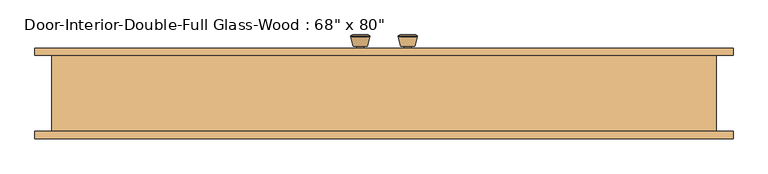
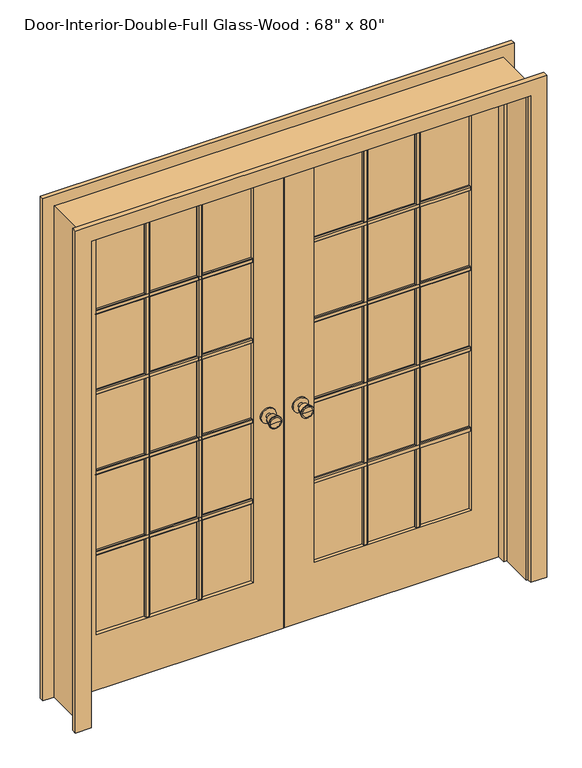
"""IFC4 building model written with IfcOpenShell, lengths in millimetres: door geometry."""

from ifc_helpers import new_model, si_unit, point, frame, frame_2d, origin, place, context, project, spatial, polyline, circle_curve, trimmed, segment, composite_curve, outline, extrude, faceted_brep, source, transform, mapped, element, save
from ifc_brep_helpers import plane_surface, cylinder_surface, revolved_surface, advanced_brep


def door_146fce4d(model_context):
    return source(origin(), model_context, "Body", "SolidModel", [
        advanced_brep(
        [(-63.5, 104.425, 914.4), (-73.5, 104.425, 914.4), (-53.5, 104.425, 914.4), (-83.9758676, 153.425, 914.4), (-63.5, 153.425, 914.4), (-43.0241324, 153.425, 914.4), (-88.5, 151.5971319, 914.4), (-38.5, 151.5971319, 914.4), (-88.5, 148.1334537, 914.4), (-38.5, 148.1334537, 914.4), (-82.136236, 123.425, 914.4), (-44.863764, 123.425, 914.4), (-73.5, 123.425, 914.4), (-53.5, 123.425, 914.4)],
        [
            (0, 1),
            (1, 2, circle_curve(frame((-63.5, 104.425, 914.4), z_axis=(0.0, -1.0, 0.0), x_axis=(1.0, 0.0, 0.0)), 10.0)),
            (2, 0),
            (2, 1, circle_curve(frame((-63.5, 104.425, 914.4), z_axis=(0.0, -1.0, 0.0), x_axis=(1.0, 0.0, 0.0)), 10.0)),
            (3, 4),
            (4, 5),
            (5, 3, circle_curve(frame((-63.5, 153.425, 914.4), z_axis=(0.0, 1.0, 0.0), x_axis=(1.0, 0.0, 0.0)), 20.4758676)),
            (3, 5, circle_curve(frame((-63.5, 153.425, 914.4), z_axis=(0.0, 1.0, 0.0), x_axis=(1.0, 0.0, 0.0)), 20.4758676)),
            (6, 3),
            (5, 7),
            (7, 6, circle_curve(frame((-63.5, 151.5971319, 914.4), z_axis=(0.0, 1.0, 0.0), x_axis=(1.0, 0.0, 0.0)), 25.0)),
            (6, 7, circle_curve(frame((-63.5, 151.5971319, 914.4), z_axis=(0.0, 1.0, 0.0), x_axis=(1.0, 0.0, 0.0)), 25.0)),
            (8, 6),
            (7, 9),
            (9, 8, circle_curve(frame((-63.5, 148.1334537, 914.4), z_axis=(0.0, 1.0, 0.0), x_axis=(1.0, 0.0, 0.0)), 25.0)),
            (8, 9, circle_curve(frame((-63.5, 148.1334537, 914.4), z_axis=(0.0, 1.0, 0.0), x_axis=(1.0, 0.0, 0.0)), 25.0)),
            (10, 8),
            (9, 11),
            (11, 10, circle_curve(frame((-63.5, 123.425, 914.4), z_axis=(0.0, 1.0, 0.0), x_axis=(1.0, 0.0, 0.0)), 18.636236)),
            (10, 11, circle_curve(frame((-63.5, 123.425, 914.4), z_axis=(0.0, 1.0, 0.0), x_axis=(1.0, 0.0, 0.0)), 18.636236)),
            (12, 10),
            (11, 13),
            (13, 12, circle_curve(frame((-63.5, 123.425, 914.4), z_axis=(0.0, 1.0, 0.0), x_axis=(1.0, 0.0, 0.0)), 10.0)),
            (12, 13, circle_curve(frame((-63.5, 123.425, 914.4), z_axis=(0.0, 1.0, 0.0), x_axis=(1.0, 0.0, 0.0)), 10.0)),
            (1, 12),
            (13, 2),
        ],
        [
            plane_surface(frame((-63.5, 104.425, 914.4), z_axis=(0.0, -1.0, 0.0), x_axis=(1.0, 0.0, 0.0))),
            plane_surface(frame((-63.5, 153.425, 914.4), z_axis=(0.0, 1.0, 0.0), x_axis=(1.0, 0.0, 0.0))),
            revolved_surface(polyline([(-43.0241324, 153.425, 914.4), (-38.5, 151.5971319, 914.4)]), (-63.5, 104.425, 914.4), (0.0, -1.0, 0.0)),
            cylinder_surface(frame((-63.5, 104.425, 914.4), z_axis=(0.0, -1.0, 0.0), x_axis=(1.0, 0.0, 0.0)), 25.0),
            revolved_surface(polyline([(-38.5, 148.1334537, 914.4), (-44.863764, 123.425, 914.4)]), (-63.5, 104.425, 914.4), (0.0, -1.0, 0.0)),
            plane_surface(frame((-63.5, 123.425, 914.4), z_axis=(0.0, -1.0, 0.0), x_axis=(1.0, 0.0, 0.0))),
            cylinder_surface(frame((-63.5, 104.425, 914.4), z_axis=(0.0, -1.0, 0.0), x_axis=(1.0, 0.0, 0.0)), 10.0),
        ],
        [
            (0, [[1, 2, 3]]),
            (0, [[-3, 4, -1]]),
            (1, [[5, 6, 7]]),
            (1, [[-6, -5, 8]]),
            (2, [[9, -7, 10, 11]]),
            (2, [[-10, -8, -9, 12]]),
            (3, [[13, -11, 14, 15]]),
            (3, [[-14, -12, -13, 16]]),
            (4, [[17, -15, 18, 19]]),
            (4, [[-18, -16, -17, 20]]),
            (5, [[21, -19, 22, 23]]),
            (5, [[-22, -20, -21, 24]]),
            (6, [[25, -23, 26, -2]]),
            (6, [[-26, -24, -25, -4]]),
        ],
    ),
        extrude(outline(composite_curve([segment(trimmed(circle_curve(frame_2d((914.4, -63.5)), 30.0), [point((914.4, -33.5))], [point((914.4, -93.5))], False, "CARTESIAN"), True, "CONTINUOUS"), segment(trimmed(circle_curve(frame_2d((914.4, -63.5)), 30.0), [point((914.4, -93.5))], [point((914.4, -33.5))], False, "CARTESIAN"), True, "CONTINUOUS")], self_intersect=False)), frame((0.0, 98.425, 0.0), z_axis=(0.0, 1.0, 0.0), x_axis=(0.0, 0.0, 1.0)), (0.0, 0.0, 1.0), 6.0),
        advanced_brep(
        [(-63.5, 57.5, 914.4), (-53.5, 57.5, 914.4), (-73.5, 57.5, 914.4), (-83.9758676, 8.5, 914.4), (-43.0241324, 8.5, 914.4), (-63.5, 8.5, 914.4), (-88.5, 10.3278681, 914.4), (-38.5, 10.3278681, 914.4), (-88.5, 13.7915463, 914.4), (-38.5, 13.7915463, 914.4), (-82.136236, 38.5, 914.4), (-44.863764, 38.5, 914.4), (-73.5, 38.5, 914.4), (-53.5, 38.5, 914.4)],
        [
            (0, 1),
            (1, 2, circle_curve(frame((-63.5, 57.5, 914.4), z_axis=(0.0, 1.0, 0.0), x_axis=(1.0, 0.0, 0.0)), 10.0)),
            (2, 0),
            (2, 1, circle_curve(frame((-63.5, 57.5, 914.4), z_axis=(0.0, 1.0, 0.0), x_axis=(1.0, 0.0, 0.0)), 10.0)),
            (3, 4, circle_curve(frame((-63.5, 8.5, 914.4), z_axis=(0.0, -1.0, 0.0), x_axis=(1.0, 0.0, 0.0)), 20.4758676)),
            (4, 5),
            (5, 3),
            (4, 3, circle_curve(frame((-63.5, 8.5, 914.4), z_axis=(0.0, -1.0, 0.0), x_axis=(1.0, 0.0, 0.0)), 20.4758676)),
            (6, 7, circle_curve(frame((-63.5, 10.3278681, 914.4), z_axis=(0.0, -1.0, 0.0), x_axis=(1.0, 0.0, 0.0)), 25.0)),
            (7, 4),
            (3, 6),
            (7, 6, circle_curve(frame((-63.5, 10.3278681, 914.4), z_axis=(0.0, -1.0, 0.0), x_axis=(1.0, 0.0, 0.0)), 25.0)),
            (8, 9, circle_curve(frame((-63.5, 13.7915463, 914.4), z_axis=(0.0, -1.0, 0.0), x_axis=(1.0, 0.0, 0.0)), 25.0)),
            (9, 7),
            (6, 8),
            (9, 8, circle_curve(frame((-63.5, 13.7915463, 914.4), z_axis=(0.0, -1.0, 0.0), x_axis=(1.0, 0.0, 0.0)), 25.0)),
            (10, 11, circle_curve(frame((-63.5, 38.5, 914.4), z_axis=(0.0, -1.0, 0.0), x_axis=(1.0, 0.0, 0.0)), 18.636236)),
            (11, 9),
            (8, 10),
            (11, 10, circle_curve(frame((-63.5, 38.5, 914.4), z_axis=(0.0, -1.0, 0.0), x_axis=(1.0, 0.0, 0.0)), 18.636236)),
            (12, 13, circle_curve(frame((-63.5, 38.5, 914.4), z_axis=(0.0, -1.0, 0.0), x_axis=(1.0, 0.0, 0.0)), 10.0)),
            (13, 11),
            (10, 12),
            (13, 12, circle_curve(frame((-63.5, 38.5, 914.4), z_axis=(0.0, -1.0, 0.0), x_axis=(1.0, 0.0, 0.0)), 10.0)),
            (1, 13),
            (12, 2),
        ],
        [
            plane_surface(frame((-63.5, 57.5, 914.4), z_axis=(0.0, 1.0, 0.0), x_axis=(1.0, 0.0, 0.0))),
            plane_surface(frame((-63.5, 8.5, 914.4), z_axis=(0.0, -1.0, 0.0), x_axis=(1.0, 0.0, 0.0))),
            revolved_surface(polyline([(-43.0241324, 8.5, 914.4), (-38.5, 10.3278681, 914.4)]), (-63.5, 57.5, 914.4), (0.0, 1.0, 0.0)),
            cylinder_surface(frame((-63.5, 57.5, 914.4), z_axis=(0.0, 1.0, 0.0), x_axis=(1.0, 0.0, 0.0)), 25.0),
            revolved_surface(polyline([(-38.5, 13.7915463, 914.4), (-44.863764, 38.5, 914.4)]), (-63.5, 57.5, 914.4), (0.0, 1.0, 0.0)),
            plane_surface(frame((-63.5, 38.5, 914.4), z_axis=(0.0, 1.0, 0.0), x_axis=(1.0, 0.0, 0.0))),
            cylinder_surface(frame((-63.5, 57.5, 914.4), z_axis=(0.0, 1.0, 0.0), x_axis=(1.0, 0.0, 0.0)), 10.0),
        ],
        [
            (0, [[1, 2, 3]]),
            (0, [[-3, 4, -1]]),
            (1, [[5, 6, 7]]),
            (1, [[8, -7, -6]]),
            (2, [[9, 10, -5, 11]]),
            (2, [[12, -11, -8, -10]]),
            (3, [[13, 14, -9, 15]]),
            (3, [[16, -15, -12, -14]]),
            (4, [[17, 18, -13, 19]]),
            (4, [[20, -19, -16, -18]]),
            (5, [[21, 22, -17, 23]]),
            (5, [[24, -23, -20, -22]]),
            (6, [[-2, 25, -21, 26]]),
            (6, [[-4, -26, -24, -25]]),
        ],
    ),
        extrude(outline(composite_curve([segment(trimmed(circle_curve(frame_2d((914.4, -63.5)), 30.0), [point((914.4, -33.5))], [point((914.4, -93.5))], False, "CARTESIAN"), True, "CONTINUOUS"), segment(trimmed(circle_curve(frame_2d((914.4, -63.5)), 30.0), [point((914.4, -93.5))], [point((914.4, -33.5))], False, "CARTESIAN"), True, "CONTINUOUS")], self_intersect=False)), frame((0.0, 57.5, 0.0), z_axis=(0.0, 1.0, 0.0), x_axis=(0.0, 0.0, 1.0)), (0.0, 0.0, 1.0), 6.0),
        extrude(outline(polyline([(77.47, 1586.23), (77.47, 1567.18), (71.12, 1567.18), (67.945, 1570.355), (67.945, 1583.055), (71.12, 1586.23), (77.47, 1586.23)])), frame((120.65, 0.0, 0.0), z_axis=(1.0, 0.0, 0.0), x_axis=(0.0, 1.0, 0.0)), (0.0, 0.0, 1.0), 622.3),
        extrude(outline(polyline([(77.47, 1249.9975), (77.47, 1230.9475), (71.12, 1230.9475), (67.945, 1234.1225), (67.945, 1246.8225), (71.12, 1249.9975), (77.47, 1249.9975)])), frame((120.65, 0.0, 0.0), z_axis=(1.0, 0.0, 0.0), x_axis=(0.0, 1.0, 0.0)), (0.0, 0.0, 1.0), 622.3),
        extrude(outline(polyline([(77.47, 913.765), (77.47, 894.715), (71.12, 894.715), (67.945, 897.89), (67.945, 910.59), (71.12, 913.765), (77.47, 913.765)])), frame((120.65, 0.0, 0.0), z_axis=(1.0, 0.0, 0.0), x_axis=(0.0, 1.0, 0.0)), (0.0, 0.0, 1.0), 622.3),
        extrude(outline(polyline([(77.47, 577.5325), (77.47, 558.4825), (71.12, 558.4825), (67.945, 561.6575), (67.945, 574.3575), (71.12, 577.5325), (77.47, 577.5325)])), frame((120.65, 0.0, 0.0), z_axis=(1.0, 0.0, 0.0), x_axis=(0.0, 1.0, 0.0)), (0.0, 0.0, 1.0), 622.3),
        extrude(outline(polyline([(525.9916667, 77.47), (545.0416667, 77.47), (545.0416667, 71.12), (541.8666667, 67.945), (529.1666667, 67.945), (525.9916667, 71.12), (525.9916667, 77.47)])), frame((0.0, 0.0, 231.775), z_axis=(0.0, 0.0, 1.0), x_axis=(1.0, 0.0, 0.0)), (0.0, 0.0, 1.0), 1681.1625),
        extrude(outline(polyline([(318.5583333, 77.47), (337.6083333, 77.47), (337.6083333, 71.12), (334.4333333, 67.945), (321.7333333, 67.945), (318.5583333, 71.12), (318.5583333, 77.47)])), frame((0.0, 0.0, 231.775), z_axis=(0.0, 0.0, 1.0), x_axis=(1.0, 0.0, 0.0)), (0.0, 0.0, 1.0), 1681.1625),
        extrude(outline(polyline([(84.455, 1586.23), (90.805, 1586.23), (93.98, 1583.055), (93.98, 1570.355), (90.805, 1567.18), (84.455, 1567.18), (84.455, 1586.23)])), frame((-742.95, 0.0, 0.0), z_axis=(1.0, 0.0, 0.0), x_axis=(0.0, 1.0, 0.0)), (0.0, 0.0, 1.0), 622.3),
        extrude(outline(polyline([(84.455, 1249.9975), (90.805, 1249.9975), (93.98, 1246.8225), (93.98, 1234.1225), (90.805, 1230.9475), (84.455, 1230.9475), (84.455, 1249.9975)])), frame((-742.95, 0.0, 0.0), z_axis=(1.0, 0.0, 0.0), x_axis=(0.0, 1.0, 0.0)), (0.0, 0.0, 1.0), 622.3),
        extrude(outline(polyline([(84.455, 913.765), (90.805, 913.765), (93.98, 910.59), (93.98, 897.89), (90.805, 894.715), (84.455, 894.715), (84.455, 913.765)])), frame((-742.95, 0.0, 0.0), z_axis=(1.0, 0.0, 0.0), x_axis=(0.0, 1.0, 0.0)), (0.0, 0.0, 1.0), 622.3),
        extrude(outline(polyline([(84.455, 577.5325), (90.805, 577.5325), (93.98, 574.3575), (93.98, 561.6575), (90.805, 558.4825), (84.455, 558.4825), (84.455, 577.5325)])), frame((-742.95, 0.0, 0.0), z_axis=(1.0, 0.0, 0.0), x_axis=(0.0, 1.0, 0.0)), (0.0, 0.0, 1.0), 622.3),
        extrude(outline(polyline([(-337.6083333, 84.455), (-337.6083333, 90.805), (-334.4333333, 93.98), (-321.7333333, 93.98), (-318.5583333, 90.805), (-318.5583333, 84.455), (-337.6083333, 84.455)])), frame((0.0, 0.0, 231.775), z_axis=(0.0, 0.0, 1.0), x_axis=(1.0, 0.0, 0.0)), (0.0, 0.0, 1.0), 1681.1625),
        extrude(outline(polyline([(-545.0416667, 84.455), (-545.0416667, 90.805), (-541.8666667, 93.98), (-529.1666667, 93.98), (-525.9916667, 90.805), (-525.9916667, 84.455), (-545.0416667, 84.455)])), frame((0.0, 0.0, 231.775), z_axis=(0.0, 0.0, 1.0), x_axis=(1.0, 0.0, 0.0)), (0.0, 0.0, 1.0), 1681.1625),
        extrude(outline(polyline([(84.455, 1586.23), (90.805, 1586.23), (93.98, 1583.055), (93.98, 1570.355), (90.805, 1567.18), (84.455, 1567.18), (84.455, 1586.23)])), frame((120.65, 0.0, 0.0), z_axis=(1.0, 0.0, 0.0), x_axis=(0.0, 1.0, 0.0)), (0.0, 0.0, 1.0), 622.3),
        extrude(outline(polyline([(84.455, 1249.9975), (90.805, 1249.9975), (93.98, 1246.8225), (93.98, 1234.1225), (90.805, 1230.9475), (84.455, 1230.9475), (84.455, 1249.9975)])), frame((120.65, 0.0, 0.0), z_axis=(1.0, 0.0, 0.0), x_axis=(0.0, 1.0, 0.0)), (0.0, 0.0, 1.0), 622.3),
        extrude(outline(polyline([(84.455, 913.765), (90.805, 913.765), (93.98, 910.59), (93.98, 897.89), (90.805, 894.715), (84.455, 894.715), (84.455, 913.765)])), frame((120.65, 0.0, 0.0), z_axis=(1.0, 0.0, 0.0), x_axis=(0.0, 1.0, 0.0)), (0.0, 0.0, 1.0), 622.3),
        extrude(outline(polyline([(84.455, 577.5325), (90.805, 577.5325), (93.98, 574.3575), (93.98, 561.6575), (90.805, 558.4825), (84.455, 558.4825), (84.455, 577.5325)])), frame((120.65, 0.0, 0.0), z_axis=(1.0, 0.0, 0.0), x_axis=(0.0, 1.0, 0.0)), (0.0, 0.0, 1.0), 622.3),
        extrude(outline(polyline([(525.9916667, 84.455), (525.9916667, 90.805), (529.1666667, 93.98), (541.8666667, 93.98), (545.0416667, 90.805), (545.0416667, 84.455), (525.9916667, 84.455)])), frame((0.0, 0.0, 231.775), z_axis=(0.0, 0.0, 1.0), x_axis=(1.0, 0.0, 0.0)), (0.0, 0.0, 1.0), 1681.1625),
        extrude(outline(polyline([(318.5583333, 84.455), (318.5583333, 90.805), (321.7333333, 93.98), (334.4333333, 93.98), (337.6083333, 90.805), (337.6083333, 84.455), (318.5583333, 84.455)])), frame((0.0, 0.0, 231.775), z_axis=(0.0, 0.0, 1.0), x_axis=(1.0, 0.0, 0.0)), (0.0, 0.0, 1.0), 1681.1625),
        extrude(outline(polyline([(77.47, 1586.23), (77.47, 1567.18), (71.12, 1567.18), (67.945, 1570.355), (67.945, 1583.055), (71.12, 1586.23), (77.47, 1586.23)])), frame((-742.95, 0.0, 0.0), z_axis=(1.0, 0.0, 0.0), x_axis=(0.0, 1.0, 0.0)), (0.0, 0.0, 1.0), 622.3),
        extrude(outline(polyline([(77.47, 1249.9975), (77.47, 1230.9475), (71.12, 1230.9475), (67.945, 1234.1225), (67.945, 1246.8225), (71.12, 1249.9975), (77.47, 1249.9975)])), frame((-742.95, 0.0, 0.0), z_axis=(1.0, 0.0, 0.0), x_axis=(0.0, 1.0, 0.0)), (0.0, 0.0, 1.0), 622.3),
        extrude(outline(polyline([(77.47, 913.765), (77.47, 894.715), (71.12, 894.715), (67.945, 897.89), (67.945, 910.59), (71.12, 913.765), (77.47, 913.765)])), frame((-742.95, 0.0, 0.0), z_axis=(1.0, 0.0, 0.0), x_axis=(0.0, 1.0, 0.0)), (0.0, 0.0, 1.0), 622.3),
        extrude(outline(polyline([(77.47, 577.5325), (77.47, 558.4825), (71.12, 558.4825), (67.945, 561.6575), (67.945, 574.3575), (71.12, 577.5325), (77.47, 577.5325)])), frame((-742.95, 0.0, 0.0), z_axis=(1.0, 0.0, 0.0), x_axis=(0.0, 1.0, 0.0)), (0.0, 0.0, 1.0), 622.3),
        extrude(outline(polyline([(-337.6083333, 77.47), (-318.5583333, 77.47), (-318.5583333, 71.12), (-321.7333333, 67.945), (-334.4333333, 67.945), (-337.6083333, 71.12), (-337.6083333, 77.47)])), frame((0.0, 0.0, 231.775), z_axis=(0.0, 0.0, 1.0), x_axis=(1.0, 0.0, 0.0)), (0.0, 0.0, 1.0), 1681.1625),
        extrude(outline(polyline([(-545.0416667, 77.47), (-525.9916667, 77.47), (-525.9916667, 71.12), (-529.1666667, 67.945), (-541.8666667, 67.945), (-545.0416667, 71.12), (-545.0416667, 77.47)])), frame((0.0, 0.0, 231.775), z_axis=(0.0, 0.0, 1.0), x_axis=(1.0, 0.0, 0.0)), (0.0, 0.0, 1.0), 1681.1625),
        advanced_brep(
        [(63.5, 57.5, 914.4), (73.5, 57.5, 914.4), (53.5, 57.5, 914.4), (83.9758676, 8.5, 914.4), (63.5, 8.5, 914.4), (43.0241324, 8.5, 914.4), (88.5, 10.3278681, 914.4), (38.5, 10.3278681, 914.4), (88.5, 13.7915463, 914.4), (38.5, 13.7915463, 914.4), (82.136236, 38.5, 914.4), (44.863764, 38.5, 914.4), (73.5, 38.5, 914.4), (53.5, 38.5, 914.4)],
        [
            (0, 1),
            (1, 2, circle_curve(frame((63.5, 57.5, 914.4), z_axis=(0.0, 1.0, 0.0), x_axis=(-1.0, 0.0, 0.0)), 10.0)),
            (2, 0),
            (2, 1, circle_curve(frame((63.5, 57.5, 914.4), z_axis=(0.0, 1.0, 0.0), x_axis=(-1.0, 0.0, 0.0)), 10.0)),
            (3, 4),
            (4, 5),
            (5, 3, circle_curve(frame((63.5, 8.5, 914.4), z_axis=(0.0, -1.0, 0.0), x_axis=(-1.0, 0.0, 0.0)), 20.4758676)),
            (3, 5, circle_curve(frame((63.5, 8.5, 914.4), z_axis=(0.0, -1.0, 0.0), x_axis=(-1.0, 0.0, 0.0)), 20.4758676)),
            (6, 3),
            (5, 7),
            (7, 6, circle_curve(frame((63.5, 10.3278681, 914.4), z_axis=(0.0, -1.0, 0.0), x_axis=(-1.0, 0.0, 0.0)), 25.0)),
            (6, 7, circle_curve(frame((63.5, 10.3278681, 914.4), z_axis=(0.0, -1.0, 0.0), x_axis=(-1.0, 0.0, 0.0)), 25.0)),
            (8, 6),
            (7, 9),
            (9, 8, circle_curve(frame((63.5, 13.7915463, 914.4), z_axis=(0.0, -1.0, 0.0), x_axis=(-1.0, 0.0, 0.0)), 25.0)),
            (8, 9, circle_curve(frame((63.5, 13.7915463, 914.4), z_axis=(0.0, -1.0, 0.0), x_axis=(-1.0, 0.0, 0.0)), 25.0)),
            (10, 8),
            (9, 11),
            (11, 10, circle_curve(frame((63.5, 38.5, 914.4), z_axis=(0.0, -1.0, 0.0), x_axis=(-1.0, 0.0, 0.0)), 18.636236)),
            (10, 11, circle_curve(frame((63.5, 38.5, 914.4), z_axis=(0.0, -1.0, 0.0), x_axis=(-1.0, 0.0, 0.0)), 18.636236)),
            (12, 10),
            (11, 13),
            (13, 12, circle_curve(frame((63.5, 38.5, 914.4), z_axis=(0.0, -1.0, 0.0), x_axis=(-1.0, 0.0, 0.0)), 10.0)),
            (12, 13, circle_curve(frame((63.5, 38.5, 914.4), z_axis=(0.0, -1.0, 0.0), x_axis=(-1.0, 0.0, 0.0)), 10.0)),
            (1, 12),
            (13, 2),
        ],
        [
            plane_surface(frame((63.5, 57.5, 914.4), z_axis=(0.0, 1.0, 0.0), x_axis=(-1.0, 0.0, 0.0))),
            plane_surface(frame((63.5, 8.5, 914.4), z_axis=(0.0, -1.0, 0.0), x_axis=(-1.0, 0.0, 0.0))),
            revolved_surface(polyline([(43.0241324, 8.5, 914.4), (38.5, 10.3278681, 914.4)]), (63.5, 57.5, 914.4), (0.0, 1.0, 0.0)),
            cylinder_surface(frame((63.5, 57.5, 914.4), z_axis=(0.0, 1.0, 0.0), x_axis=(-1.0, 0.0, 0.0)), 25.0),
            revolved_surface(polyline([(38.5, 13.7915463, 914.4), (44.863764, 38.5, 914.4)]), (63.5, 57.5, 914.4), (0.0, 1.0, 0.0)),
            plane_surface(frame((63.5, 38.5, 914.4), z_axis=(0.0, 1.0, 0.0), x_axis=(-1.0, 0.0, 0.0))),
            cylinder_surface(frame((63.5, 57.5, 914.4), z_axis=(0.0, 1.0, 0.0), x_axis=(-1.0, 0.0, 0.0)), 10.0),
        ],
        [
            (0, [[1, 2, 3]]),
            (0, [[-3, 4, -1]]),
            (1, [[5, 6, 7]]),
            (1, [[-6, -5, 8]]),
            (2, [[9, -7, 10, 11]]),
            (2, [[-10, -8, -9, 12]]),
            (3, [[13, -11, 14, 15]]),
            (3, [[-14, -12, -13, 16]]),
            (4, [[17, -15, 18, 19]]),
            (4, [[-18, -16, -17, 20]]),
            (5, [[21, -19, 22, 23]]),
            (5, [[-22, -20, -21, 24]]),
            (6, [[25, -23, 26, -2]]),
            (6, [[-26, -24, -25, -4]]),
        ],
    ),
        extrude(outline(composite_curve([segment(trimmed(circle_curve(frame_2d((914.4, 63.5)), 30.0), [point((914.4, 33.5))], [point((914.4, 93.5))], False, "CARTESIAN"), True, "CONTINUOUS"), segment(trimmed(circle_curve(frame_2d((914.4, 63.5)), 30.0), [point((914.4, 93.5))], [point((914.4, 33.5))], False, "CARTESIAN"), True, "CONTINUOUS")], self_intersect=False)), frame((0.0, 57.5, 0.0), z_axis=(0.0, 1.0, 0.0), x_axis=(0.0, 0.0, 1.0)), (0.0, 0.0, 1.0), 6.0),
        advanced_brep(
        [(63.5, 104.425, 914.4), (53.5, 104.425, 914.4), (73.5, 104.425, 914.4), (83.9758676, 153.425, 914.4), (43.0241324, 153.425, 914.4), (63.5, 153.425, 914.4), (88.5, 151.5971319, 914.4), (38.5, 151.5971319, 914.4), (88.5, 148.1334537, 914.4), (38.5, 148.1334537, 914.4), (82.136236, 123.425, 914.4), (44.863764, 123.425, 914.4), (73.5, 123.425, 914.4), (53.5, 123.425, 914.4)],
        [
            (0, 1),
            (1, 2, circle_curve(frame((63.5, 104.425, 914.4), z_axis=(0.0, -1.0, 0.0), x_axis=(-1.0, 0.0, 0.0)), 10.0)),
            (2, 0),
            (2, 1, circle_curve(frame((63.5, 104.425, 914.4), z_axis=(0.0, -1.0, 0.0), x_axis=(-1.0, 0.0, 0.0)), 10.0)),
            (3, 4, circle_curve(frame((63.5, 153.425, 914.4), z_axis=(0.0, 1.0, 0.0), x_axis=(-1.0, 0.0, 0.0)), 20.4758676)),
            (4, 5),
            (5, 3),
            (4, 3, circle_curve(frame((63.5, 153.425, 914.4), z_axis=(0.0, 1.0, 0.0), x_axis=(-1.0, 0.0, 0.0)), 20.4758676)),
            (6, 7, circle_curve(frame((63.5, 151.5971319, 914.4), z_axis=(0.0, 1.0, 0.0), x_axis=(-1.0, 0.0, 0.0)), 25.0)),
            (7, 4),
            (3, 6),
            (7, 6, circle_curve(frame((63.5, 151.5971319, 914.4), z_axis=(0.0, 1.0, 0.0), x_axis=(-1.0, 0.0, 0.0)), 25.0)),
            (8, 9, circle_curve(frame((63.5, 148.1334537, 914.4), z_axis=(0.0, 1.0, 0.0), x_axis=(-1.0, 0.0, 0.0)), 25.0)),
            (9, 7),
            (6, 8),
            (9, 8, circle_curve(frame((63.5, 148.1334537, 914.4), z_axis=(0.0, 1.0, 0.0), x_axis=(-1.0, 0.0, 0.0)), 25.0)),
            (10, 11, circle_curve(frame((63.5, 123.425, 914.4), z_axis=(0.0, 1.0, 0.0), x_axis=(-1.0, 0.0, 0.0)), 18.636236)),
            (11, 9),
            (8, 10),
            (11, 10, circle_curve(frame((63.5, 123.425, 914.4), z_axis=(0.0, 1.0, 0.0), x_axis=(-1.0, 0.0, 0.0)), 18.636236)),
            (12, 13, circle_curve(frame((63.5, 123.425, 914.4), z_axis=(0.0, 1.0, 0.0), x_axis=(-1.0, 0.0, 0.0)), 10.0)),
            (13, 11),
            (10, 12),
            (13, 12, circle_curve(frame((63.5, 123.425, 914.4), z_axis=(0.0, 1.0, 0.0), x_axis=(-1.0, 0.0, 0.0)), 10.0)),
            (1, 13),
            (12, 2),
        ],
        [
            plane_surface(frame((63.5, 104.425, 914.4), z_axis=(0.0, -1.0, 0.0), x_axis=(-1.0, 0.0, 0.0))),
            plane_surface(frame((63.5, 153.425, 914.4), z_axis=(0.0, 1.0, 0.0), x_axis=(-1.0, 0.0, 0.0))),
            revolved_surface(polyline([(43.0241324, 153.425, 914.4), (38.5, 151.5971319, 914.4)]), (63.5, 104.425, 914.4), (0.0, -1.0, 0.0)),
            cylinder_surface(frame((63.5, 104.425, 914.4), z_axis=(0.0, -1.0, 0.0), x_axis=(-1.0, 0.0, 0.0)), 25.0),
            revolved_surface(polyline([(38.5, 148.1334537, 914.4), (44.863764, 123.425, 914.4)]), (63.5, 104.425, 914.4), (0.0, -1.0, 0.0)),
            plane_surface(frame((63.5, 123.425, 914.4), z_axis=(0.0, -1.0, 0.0), x_axis=(-1.0, 0.0, 0.0))),
            cylinder_surface(frame((63.5, 104.425, 914.4), z_axis=(0.0, -1.0, 0.0), x_axis=(-1.0, 0.0, 0.0)), 10.0),
        ],
        [
            (0, [[1, 2, 3]]),
            (0, [[-3, 4, -1]]),
            (1, [[5, 6, 7]]),
            (1, [[8, -7, -6]]),
            (2, [[9, 10, -5, 11]]),
            (2, [[12, -11, -8, -10]]),
            (3, [[13, 14, -9, 15]]),
            (3, [[16, -15, -12, -14]]),
            (4, [[17, 18, -13, 19]]),
            (4, [[20, -19, -16, -18]]),
            (5, [[21, 22, -17, 23]]),
            (5, [[24, -23, -20, -22]]),
            (6, [[-2, 25, -21, 26]]),
            (6, [[-4, -26, -24, -25]]),
        ],
    ),
        extrude(outline(composite_curve([segment(trimmed(circle_curve(frame_2d((914.4, 63.5)), 30.0), [point((914.4, 33.5))], [point((914.4, 93.5))], False, "CARTESIAN"), True, "CONTINUOUS"), segment(trimmed(circle_curve(frame_2d((914.4, 63.5)), 30.0), [point((914.4, 93.5))], [point((914.4, 33.5))], False, "CARTESIAN"), True, "CONTINUOUS")], self_intersect=False)), frame((0.0, 98.425, 0.0), z_axis=(0.0, 1.0, 0.0), x_axis=(0.0, 0.0, 1.0)), (0.0, 0.0, 1.0), 6.0),
        extrude(outline(polyline([(0.0, 869.95), (0.0, 933.45), (2101.85, 933.45), (2101.85, -933.45), (0.0, -933.45), (0.0, -869.95), (2038.35, -869.95), (2038.35, 869.95), (0.0, 869.95)])), frame((0.0, 98.425, 0.0), z_axis=(0.0, 1.0, 0.0), x_axis=(0.0, 0.0, 1.0)), (0.0, 0.0, 1.0), 19.05),
        extrude(outline(polyline([(0.0, 869.95), (0.0, 933.45), (2101.85, 933.45), (2101.85, -933.45), (0.0, -933.45), (0.0, -869.95), (2038.35, -869.95), (2038.35, 869.95), (0.0, 869.95)])), frame((0.0, -123.825, 0.0), z_axis=(0.0, 1.0, 0.0), x_axis=(0.0, 0.0, 1.0)), (0.0, 0.0, 1.0), 19.05),
        extrude(outline(polyline([(2032.0, -863.6), (0.0, -863.6), (0.0, -1.6019111), (2032.0, -1.6019111), (2032.0, -863.6)]), holes=[polyline([(231.775, -742.95), (1912.9375, -742.95), (1912.9375, -120.65), (231.775, -120.65), (231.775, -742.95)])]), frame((0.0, 63.5, 0.0), z_axis=(0.0, 1.0, 0.0), x_axis=(0.0, 0.0, 1.0)), (0.0, 0.0, 1.0), 34.925),
        extrude(outline(polyline([(0.0, 863.6), (2032.0, 863.6), (2032.0, 1.5875), (0.0, 1.5875), (0.0, 863.6)]), holes=[polyline([(1912.9375, 120.65), (1912.9375, 742.95), (231.775, 742.95), (231.775, 120.65), (1912.9375, 120.65)])]), frame((0.0, 63.5, 0.0), z_axis=(0.0, 1.0, 0.0), x_axis=(0.0, 0.0, 1.0)), (0.0, 0.0, 1.0), 34.925),
        faceted_brep([(889.0, 98.425, 0.0), (889.0, -104.775, 0.0), (863.6, -104.775, 0.0), (863.6, 28.575, 0.0), (850.9, 28.575, 0.0), (850.9, 63.5, 0.0), (863.6, 63.5, 0.0), (863.6, 98.425, 0.0), (889.0, 98.425, 2057.4), (889.0, -104.775, 2057.4), (-889.0, -104.775, 2057.4), (-889.0, -104.775, 0.0), (-863.6, -104.775, 0.0), (-863.6, -104.775, 2032.0), (863.6, -104.775, 2032.0), (863.6, 28.575, 2032.0), (-863.6, 28.575, 2032.0), (-863.6, 28.575, 0.0), (-850.9, 28.575, 0.0), (-850.9, 28.575, 2019.3), (850.9, 28.575, 2019.3), (850.9, 63.5, 2019.3), (1.5875, 63.5, 2019.3), (-1.6019111, 63.5, 2019.3), (-850.9, 63.5, 2019.3), (-850.9, 63.5, 0.0), (-863.6, 63.5, 0.0), (-863.6, 63.5, 2032.0), (-1.6019111, 63.5, 2032.0), (1.5875, 63.5, 2032.0), (863.6, 63.5, 2032.0), (863.6, 98.425, 2032.0), (1.5875, 98.425, 2032.0), (-1.6019111, 98.425, 2032.0), (-863.6, 98.425, 2032.0), (-863.6, 98.425, 0.0), (-889.0, 98.425, 0.0), (-889.0, 98.425, 2057.4)], [[[0, 1, 2, 3, 4, 5, 6, 7]], [[1, 0, 8, 9]], [[2, 1, 9, 10, 11, 12, 13, 14]], [[3, 2, 14, 15]], [[4, 3, 15, 16, 17, 18, 19, 20]], [[5, 4, 20, 21]], [[6, 5, 21, 22, 23, 24, 25, 26, 27, 28, 29, 30]], [[7, 6, 30, 31]], [[0, 7, 31, 32, 33, 34, 35, 36, 37, 8]], [[9, 8, 37, 10]], [[14, 13, 16, 15]], [[20, 19, 24, 23, 22, 21]], [[31, 30, 29, 28, 27, 34, 33, 32]], [[12, 11, 36, 35, 26, 25, 18, 17]], [[11, 10, 37, 36]], [[13, 12, 17, 16]], [[19, 18, 25, 24]], [[27, 26, 35, 34]]]),
        extrude(outline(polyline([(742.95, 77.47), (120.65, 77.47), (120.65, 84.455), (742.95, 84.455), (742.95, 77.47)])), frame((0.0, 0.0, 231.775), z_axis=(0.0, 0.0, 1.0), x_axis=(1.0, 0.0, 0.0)), (0.0, 0.0, 1.0), 1681.1625),
        extrude(outline(polyline([(-120.65, 77.47), (-742.95, 77.47), (-742.95, 84.455), (-120.65, 84.455), (-120.65, 77.47)])), frame((0.0, 0.0, 231.775), z_axis=(0.0, 0.0, 1.0), x_axis=(1.0, 0.0, 0.0)), (0.0, 0.0, 1.0), 1681.1625),
    ])


if __name__ == "__main__":
    model = new_model("IFC4")
    model_context = context("Model", 3, world=origin())
    ifc_project = project(units=[si_unit("LENGTHUNIT", "METRE", prefix="MILLI")], contexts=[model_context])
    site = spatial("IfcSite", under=ifc_project)
    building = spatial("IfcBuilding", under=site)
    placement = place(None, origin())
    door_shape = door_146fce4d(model_context)
    element("IfcDoor", 1, ObjectType="Door-Interior-Double-Full Glass-Wood : 68\" x 80\"", at=placement, inside=building, context=model_context, shape_type="MappedRepresentation", body=[
        mapped(door_shape, transform((0.0, 0.0, 0.0), x_axis=(1.0, 0.0, 0.0), y_axis=(0.0, 1.0, 0.0), z_axis=(0.0, 0.0, 1.0))),
    ])
    save(model, "model.ifc")

# Revit data of these elements
# Type "Door-Interior-Double-Full Glass-Wood : 68\" x 80\""
#   Type Mark = "21"
#   Assembly Code = "C1020300"
#   Analytic Construction = "French door, wood frame with single glass"
#   Top Rail = 0' - 4 11/16"
#   Thickness = 0' - 1 3/8"
#   Thermal Resistance (R) = 1.0696 (h·ft²·°F)/BTU
#   Swing Angle [instance default] = 90.00°
#   Stiles = 0' - 4 3/4"
#   Rough Width = 5' - 10"
#   Rough Height = 6' - 9"
#   Panel Width = 2' - 10"
#   Height = 6' - 8"
#   Width = 5' - 8"
#   Heat Transfer Coefficient (U) = 0.9350 BTU/(h·ft²·°F)
#   Bottom Rail = 0' - 9 1/8"
#   Show Grill [instance default] = yes
#   Trim Material = Cherry
#   Panel Material = Cherry
#   Frame Material = Cherry
#   Door Handle Material = Aluminum
#   Visual Light Transmittance = 0
#   Solar Heat Gain Coefficient = 0
#   Wall Closure = (empty or 0)
#   Function = (empty or 0)
# Element 1 (IfcDoor, "Door-Interior-Double-Full Glass-Wood : 68\" x 80\"")
#   Materials on its faces: "Cherry", "Aluminum", "Glass"
# Materials
#   "Cherry": class "Wood", colour RGB 226 177 128, transparency 0, Description = "Prunus Serotina", Cost = 0
#   "Aluminum": class "Metal", colour RGB 247 247 247, transparency 0, Description = "Aluminum 6061", Cost = 0
#   "Glass": class "Glass", colour RGB 0 128 192, transparency 0.75, Description = "Soda Lime Glass", Cost = 0
